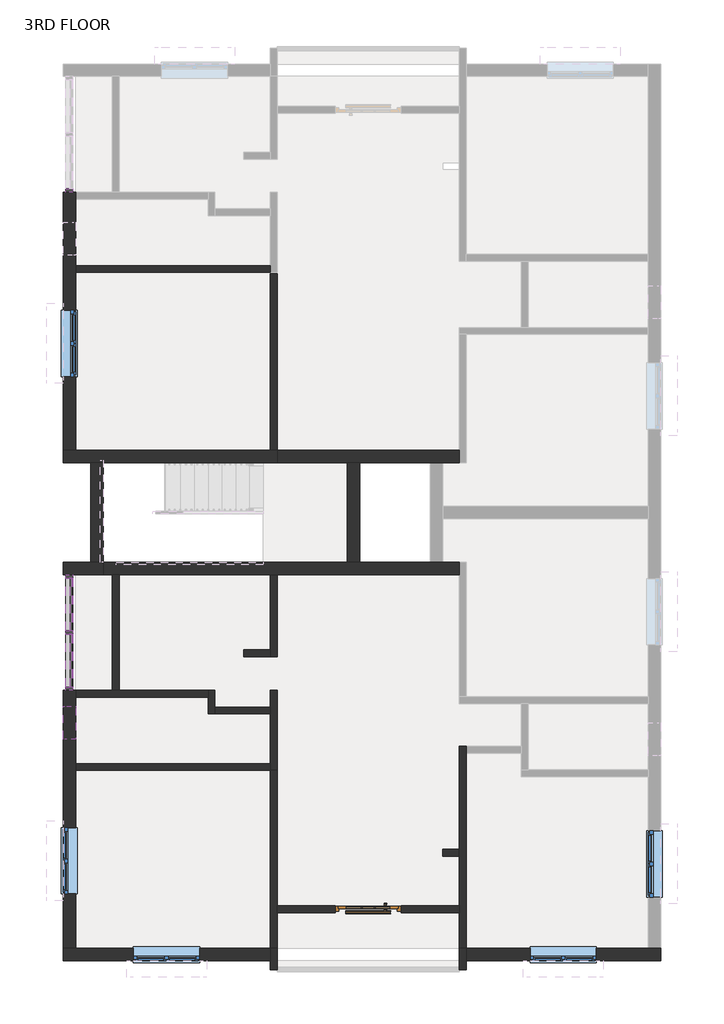
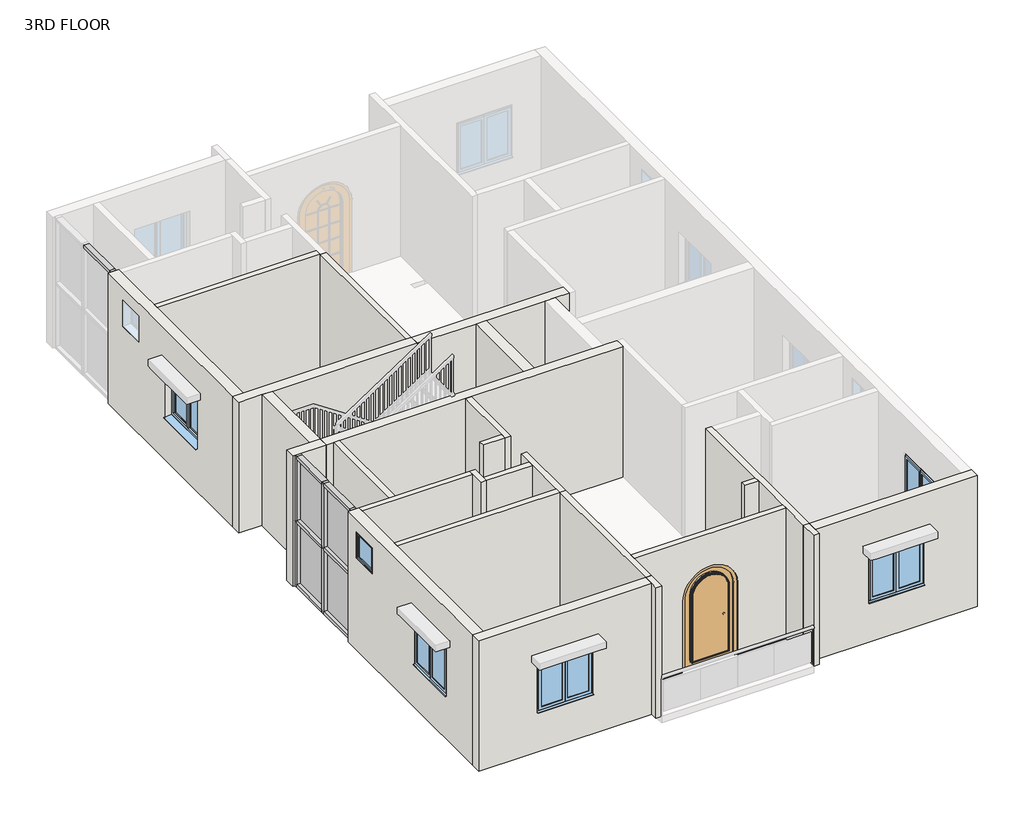
# One storey, part 1 of 4: 26 walls, 15 members, 6 windows, 4 plates, 1 door.
"""IFC4 building model written with IfcOpenShell, lengths in millimetres."""

from ifc_helpers import new_model, si_unit, point, frame, frame_2d, origin, place, context, project, spatial, polyline, circle_curve, trimmed, segment, composite_curve, outline, extrude, faceted_brep, transform, mapped, element, save
from components import door_arched_single_french_glass_wood_exterior_4_x_7_french_5c4dec95, member_801a2072, member_82905deb, member_88aa5c81, member_4491d118, system_panel_glazed_a8655be6, window_80340324, w2_windows_4_x_4_9dec5fc7

model = new_model("IFC4")

# Units and contexts
model_context = context("Model", 3, world=origin())
ifc_project = project(units=[si_unit("LENGTHUNIT", "METRE", prefix="MILLI")], contexts=[model_context])

# Site, building, storey
site = spatial("IfcSite", under=ifc_project)
building = spatial("IfcBuilding", under=site)
storey = spatial("IfcBuildingStorey", under=building, Name="3RD FLOOR", Elevation=12192.0)

# Door
placement = place(None, origin())
door_arched_single_french_glass_wood_exterior_4_x_7_french_shape = door_arched_single_french_glass_wood_exterior_4_x_7_french_5c4dec95(model_context)
element("IfcDoor", 1, ObjectType="Door_Arched_Single_French_Glass_Wood_Exterior : 4' x 7' french door", at=placement, inside=storey, context=model_context, shape_type="MappedRepresentation", body=[
    mapped(door_arched_single_french_glass_wood_exterior_4_x_7_french_shape, transform((-817.6012202, -2286.2690997, 12192.0), x_axis=(-1.0, 0.0, 0.0), y_axis=(0.0, -1.0, 0.0), z_axis=(0.0, 0.0, 1.0))),
])

# Members
member_shape = member_801a2072(model_context)
element("IfcMember", 2, ObjectType="Rectangular Mullion : 2.5\" x 5\" rectangular", at=placement, inside=storey, context=model_context, shape_type="MappedRepresentation", body=[
    mapped(member_shape, transform((-6318.2887202, 10972.5309003, 15240.0), x_axis=(0.0, 0.0, 1.0), y_axis=(-1.0, 0.0, 0.0), z_axis=(0.0, -1.0, 0.0))),
])
element("IfcMember", 3, ObjectType="Rectangular Mullion : 2.5\" x 5\" rectangular", at=placement, inside=storey, context=model_context, shape_type="MappedRepresentation", body=[
    mapped(member_shape, transform((-6318.2887202, 1803.1309003, 15240.0), x_axis=(0.0, 0.0, 1.0), y_axis=(-1.0, 0.0, 0.0), z_axis=(0.0, -1.0, 0.0))),
])
element("IfcMember", 4, ObjectType="Rectangular Mullion : 2.5\" x 5\" rectangular", at=placement, inside=storey, context=model_context, shape_type="MappedRepresentation", body=[
    mapped(member_shape, transform((-6318.2887202, 2838.1809003, 15240.0), x_axis=(0.0, 0.0, 1.0), y_axis=(-1.0, 0.0, 0.0), z_axis=(0.0, -1.0, 0.0))),
])
element("IfcMember", 5, ObjectType="Rectangular Mullion : 2.5\" x 5\" rectangular", at=placement, inside=storey, context=model_context, shape_type="MappedRepresentation", body=[
    mapped(member_shape, transform((-6318.2887202, 3809.7309003, 12192.0), x_axis=(0.0, 0.0, -1.0), y_axis=(-1.0, 0.0, 0.0), z_axis=(0.0, 1.0, 0.0))),
])
element("IfcMember", 6, ObjectType="Rectangular Mullion : 2.5\" x 5\" rectangular", at=placement, inside=storey, context=model_context, shape_type="MappedRepresentation", body=[
    mapped(member_shape, transform((-6318.2887202, 2774.6809003, 12192.0), x_axis=(0.0, 0.0, -1.0), y_axis=(-1.0, 0.0, 0.0), z_axis=(0.0, 1.0, 0.0))),
])
member_2_shape = member_82905deb(model_context)
element("IfcMember", 7, ObjectType="Rectangular Mullion : 2.5\" x 5\" rectangular", at=placement, inside=storey, context=model_context, shape_type="MappedRepresentation", body=[
    mapped(member_2_shape, transform((-6318.2887202, 2806.4309003, 12192.0), x_axis=(0.0, -1.0, 0.0), y_axis=(-1.0, 0.0, 0.0), z_axis=(0.0, 0.0, -1.0))),
])
member_3_shape = member_88aa5c81(model_context)
element("IfcMember", 8, ObjectType="Rectangular Mullion : 2.5\" x 5\" rectangular", at=placement, inside=storey, context=model_context, shape_type="MappedRepresentation", body=[
    mapped(member_3_shape, transform((-6318.2887202, 2838.1809003, 13716.0), x_axis=(0.0, 0.0, 1.0), y_axis=(-1.0, 0.0, 0.0), z_axis=(0.0, -1.0, 0.0))),
])
element("IfcMember", 9, ObjectType="Rectangular Mullion : 2.5\" x 5\" rectangular", at=placement, inside=storey, context=model_context, shape_type="MappedRepresentation", body=[
    mapped(member_3_shape, transform((-6318.2887202, 1803.1309003, 13716.0), x_axis=(0.0, 0.0, 1.0), y_axis=(-1.0, 0.0, 0.0), z_axis=(0.0, -1.0, 0.0))),
])
element("IfcMember", 10, ObjectType="Rectangular Mullion : 2.5\" x 5\" rectangular", at=placement, inside=storey, context=model_context, shape_type="MappedRepresentation", body=[
    mapped(member_2_shape, transform((-6318.2887202, 2806.4309003, 13716.0), x_axis=(0.0, -1.0, 0.0), y_axis=(-1.0, 0.0, 0.0), z_axis=(0.0, 0.0, -1.0))),
])
member_4_shape = member_4491d118(model_context)
element("IfcMember", 11, ObjectType="Rectangular Mullion : 2.5\" x 5\" rectangular", at=placement, inside=storey, context=model_context, shape_type="MappedRepresentation", body=[
    mapped(member_4_shape, transform((-6318.2887202, 10909.0309003, 12192.0), x_axis=(0.0, -1.0, 0.0), y_axis=(-1.0, 0.0, 0.0), z_axis=(0.0, 0.0, -1.0))),
])
element("IfcMember", 12, ObjectType="Rectangular Mullion : 2.5\" x 5\" rectangular", at=placement, inside=storey, context=model_context, shape_type="MappedRepresentation", body=[
    mapped(member_4_shape, transform((-6318.2887202, 1739.6309003, 12192.0), x_axis=(0.0, -1.0, 0.0), y_axis=(-1.0, 0.0, 0.0), z_axis=(0.0, 0.0, -1.0))),
])
element("IfcMember", 13, ObjectType="Rectangular Mullion : 2.5\" x 5\" rectangular", at=placement, inside=storey, context=model_context, shape_type="MappedRepresentation", body=[
    mapped(member_4_shape, transform((-6318.2887202, 3873.2309003, 15240.0), x_axis=(0.0, 1.0, 0.0), y_axis=(-1.0, 0.0, 0.0), z_axis=(0.0, 0.0, 1.0))),
])
element("IfcMember", 14, ObjectType="Rectangular Mullion : 2.5\" x 5\" rectangular", at=placement, inside=storey, context=model_context, shape_type="MappedRepresentation", body=[
    mapped(member_4_shape, transform((-6318.2887202, 10909.0309003, 13716.0), x_axis=(0.0, -1.0, 0.0), y_axis=(-1.0, 0.0, 0.0), z_axis=(0.0, 0.0, -1.0))),
])
element("IfcMember", 15, ObjectType="Rectangular Mullion : 2.5\" x 5\" rectangular", at=placement, inside=storey, context=model_context, shape_type="MappedRepresentation", body=[
    mapped(member_4_shape, transform((-6318.2887202, 1739.6309003, 13716.0), x_axis=(0.0, -1.0, 0.0), y_axis=(-1.0, 0.0, 0.0), z_axis=(0.0, 0.0, -1.0))),
])
element("IfcMember", 16, ObjectType="Rectangular Mullion : 2.5\" x 5\" rectangular", at=placement, inside=storey, context=model_context, shape_type="MappedRepresentation", body=[
    mapped(member_4_shape, transform((-6318.2887202, 3873.2309003, 13716.0), x_axis=(0.0, 1.0, 0.0), y_axis=(-1.0, 0.0, 0.0), z_axis=(0.0, 0.0, 1.0))),
])

# Plates
system_panel_glazed_shape = system_panel_glazed_a8655be6(model_context)
element("IfcPlate", 17, ObjectType="System Panel : Glazed", at=placement, inside=storey, context=model_context, shape_type="MappedRepresentation", body=[
    mapped(system_panel_glazed_shape, transform((-6318.2887202, 3323.9559003, 12255.5), x_axis=(0.0, -1.0, 0.0), y_axis=(1.0, 0.0, 0.0), z_axis=(0.0, 0.0, 1.0))),
])
element("IfcPlate", 18, ObjectType="System Panel : Glazed", at=placement, inside=storey, context=model_context, shape_type="MappedRepresentation", body=[
    mapped(system_panel_glazed_shape, transform((-6318.2887202, 2288.9059003, 12255.5), x_axis=(0.0, -1.0, 0.0), y_axis=(1.0, 0.0, 0.0), z_axis=(0.0, 0.0, 1.0))),
])
element("IfcPlate", 19, ObjectType="System Panel : Glazed", at=placement, inside=storey, context=model_context, shape_type="MappedRepresentation", body=[
    mapped(system_panel_glazed_shape, transform((-6318.2887202, 3323.9559003, 13747.75), x_axis=(0.0, -1.0, 0.0), y_axis=(1.0, 0.0, 0.0), z_axis=(0.0, 0.0, 1.0))),
])
element("IfcPlate", 20, ObjectType="System Panel : Glazed", at=placement, inside=storey, context=model_context, shape_type="MappedRepresentation", body=[
    mapped(system_panel_glazed_shape, transform((-6318.2887202, 2288.9059003, 13747.75), x_axis=(0.0, -1.0, 0.0), y_axis=(1.0, 0.0, 0.0), z_axis=(0.0, 0.0, 1.0))),
])

# Walls
element("IfcWall", 21, ObjectType="OUTER WALL 9\"", at=placement, inside=storey, context=model_context, shape_type="Brep", body=[
    faceted_brep([(-6432.5887202, -3238.7690997, 12192.0), (-2621.0012202, -3238.7690997, 12192.0), (-2621.0012202, -3238.7690997, 15240.0), (-6432.5887202, -3238.7690997, 15240.0), (-5137.1887202, -3238.7690997, 13106.4), (-5137.1887202, -3238.7690997, 14325.6), (-3917.9887202, -3238.7690997, 14325.6), (-3917.9887202, -3238.7690997, 13106.4), (-6432.5887202, -3010.1690997, 12192.0), (-6432.5887202, -3010.1690997, 15240.0), (-6203.9887202, -3010.1690997, 15240.0), (-2621.0012202, -3010.1690997, 15240.0), (-2621.0012202, -3010.1690997, 12192.0), (-6203.9887202, -3010.1690997, 12192.0), (-5137.1887202, -3010.1690997, 13106.4), (-3917.9887202, -3010.1690997, 13106.4), (-3917.9887202, -3010.1690997, 14325.6), (-5137.1887202, -3010.1690997, 14325.6)], [[[0, 1, 2, 3], [4, 5, 6, 7]], [[8, 9, 10, 11, 12, 13], [14, 15, 16, 17]], [[1, 0, 8, 13, 12]], [[3, 2, 11, 10, 9]], [[0, 3, 9, 8]], [[2, 1, 12, 11]], [[5, 4, 14, 17]], [[6, 5, 17, 16]], [[7, 6, 16, 15]], [[4, 7, 15, 14]]]),
])
element("IfcWall", 22, ObjectType="OUTER WALL 9\"", at=placement, inside=storey, context=model_context, shape_type="Brep", body=[
    faceted_brep([(-6203.9887202, -3010.1690997, 15240.0), (-6203.9887202, -3010.1690997, 12192.0), (-6203.9887202, 266.4309003, 12192.0), (-6203.9887202, 393.4309003, 12192.0), (-6203.9887202, 1612.6309003, 12192.0), (-6203.9887202, 1739.6309003, 12192.0), (-6203.9887202, 1739.6309003, 15240.0), (-6203.9887202, 1612.6309003, 15240.0), (-6203.9887202, 393.4309003, 15240.0), (-6203.9887202, 266.4309003, 15240.0), (-6203.9887202, -787.6690997, 13192.0), (-6203.9887202, -2006.8690997, 13192.0), (-6203.9887202, -2006.8690997, 14411.2), (-6203.9887202, -787.6690997, 14411.2), (-6203.9887202, 1447.5309003, 14935.2), (-6203.9887202, 1447.5309003, 14325.6), (-6203.9887202, 837.9309003, 14325.6), (-6203.9887202, 837.9309003, 14935.2), (-6432.5887202, -3010.1690997, 12192.0), (-6432.5887202, -3010.1690997, 15240.0), (-6432.5887202, 1739.6309003, 15240.0), (-6432.5887202, 1739.6309003, 12192.0), (-6432.5887202, -787.6690997, 13192.0), (-6432.5887202, -787.6690997, 14411.2), (-6432.5887202, -2006.8690997, 14411.2), (-6432.5887202, -2006.8690997, 13192.0), (-6432.5887202, 1447.5309003, 14935.2), (-6432.5887202, 837.9309003, 14935.2), (-6432.5887202, 837.9309003, 14325.6), (-6432.5887202, 1447.5309003, 14325.6)], [[[0, 1, 2, 3, 4, 5, 6, 7, 8, 9], [10, 11, 12, 13], [14, 15, 16, 17]], [[18, 19, 20, 21], [22, 23, 24, 25], [26, 27, 28, 29]], [[1, 18, 21, 5, 4, 3, 2]], [[19, 0, 9, 8, 7, 6, 20]], [[1, 0, 19, 18]], [[6, 5, 21, 20]], [[23, 22, 10, 13]], [[24, 23, 13, 12]], [[25, 24, 12, 11]], [[22, 25, 11, 10]], [[15, 14, 26, 29]], [[16, 15, 29, 28]], [[17, 16, 28, 27]], [[14, 17, 27, 26]]]),
])
element("IfcWall", 23, ObjectType="OUTER WALL 9\"", at=placement, inside=storey, context=model_context, shape_type="Brep", body=[
    faceted_brep([(4567.1987798, -3010.1690997, 12192.0), (4338.5987798, -3010.1690997, 12192.0), (985.7987798, -3010.1690997, 12192.0), (985.7987798, -3010.1690997, 15240.0), (4338.5987798, -3010.1690997, 15240.0), (4567.1987798, -3010.1690997, 15240.0), (2166.8987798, -3010.1690997, 13106.4), (3386.0987798, -3010.1690997, 13106.4), (3386.0987798, -3010.1690997, 14325.6), (2166.8987798, -3010.1690997, 14325.6), (4567.1987798, -3238.7690997, 12192.0), (4567.1987798, -3238.7690997, 15240.0), (985.7987798, -3238.7690997, 15240.0), (985.7987798, -3238.7690997, 12192.0), (2166.8987798, -3238.7690997, 13106.4), (2166.8987798, -3238.7690997, 14325.6), (3386.0987798, -3238.7690997, 14325.6), (3386.0987798, -3238.7690997, 13106.4)], [[[0, 1, 2, 3, 4, 5], [6, 7, 8, 9]], [[10, 11, 12, 13], [14, 15, 16, 17]], [[2, 1, 0, 10, 13]], [[5, 4, 3, 12, 11]], [[0, 5, 11, 10]], [[15, 14, 6, 9]], [[16, 15, 9, 8]], [[17, 16, 8, 7]], [[14, 17, 7, 6]], [[3, 2, 13, 12]]]),
])
element("IfcWall", 24, ObjectType="OUTER WALL 9\"", at=placement, inside=storey, context=model_context, shape_type="SweptSolid", body=[
    extrude(outline(polyline([(6159.2309003, 12192.0), (6159.2309003, 15240.0), (10909.0309003, 15240.0), (10909.0309003, 12192.0), (6159.2309003, 12192.0)]), holes=[polyline([(7518.1309003, 13192.0), (8737.3309003, 13192.0), (8737.3309003, 14411.2), (7518.1309003, 14411.2), (7518.1309003, 13192.0)]), polyline([(9753.3309003, 14935.2), (9753.3309003, 14325.6), (10362.9309003, 14325.6), (10362.9309003, 14935.2), (9753.3309003, 14935.2)])]), frame((-6432.5887202, 0.0, 0.0), z_axis=(1.0, 0.0, 0.0), x_axis=(0.0, 1.0, 0.0)), (0.0, 0.0, 1.0), 228.6),
])
element("IfcWall", 25, ObjectType="OUTER WALL 9\"", at=placement, inside=storey, context=model_context, shape_type="Brep", body=[
    faceted_brep([(-6432.5887202, 5930.6309003, 12192.0), (-5923.0012202, 5930.6309003, 12192.0), (-5694.4012202, 5930.6309003, 12192.0), (-2494.0012202, 5930.6309003, 12192.0), (-2494.0012202, 5930.6309003, 15240.0), (-5694.4012202, 5930.6309003, 15240.0), (-5923.0012202, 5930.6309003, 15240.0), (-6432.5887202, 5930.6309003, 15240.0), (-6432.5887202, 6159.2309003, 12192.0), (-6432.5887202, 6159.2309003, 15240.0), (-6203.9887202, 6159.2309003, 15240.0), (-2621.0012202, 6159.2309003, 15240.0), (-2494.0012202, 6159.2309003, 15240.0), (-2494.0012202, 6159.2309003, 12192.0), (-2621.0012202, 6159.2309003, 12192.0), (-6203.9887202, 6159.2309003, 12192.0)], [[[0, 1, 2, 3, 4, 5, 6, 7]], [[8, 9, 10, 11, 12, 13, 14, 15]], [[3, 2, 1, 0, 8, 15, 14, 13]], [[7, 6, 5, 4, 12, 11, 10, 9]], [[0, 7, 9, 8]], [[4, 3, 13, 12]]]),
])
element("IfcWall", 26, ObjectType="OUTER WALL 9\"", at=placement, inside=storey, context=model_context, shape_type="SweptSolid", body=[
    extrude(outline(polyline([(-5923.0012202, 4101.8309003), (-5923.0012202, 5930.6309003), (-5694.4012202, 5930.6309003), (-5694.4012202, 4101.8309003), (-5923.0012202, 4101.8309003)])), frame((0.0, 0.0, 12192.0), z_axis=(0.0, 0.0, 1.0), x_axis=(1.0, 0.0, 0.0)), (0.0, 0.0, 1.0), 3048.0),
])
element("IfcWall", 27, ObjectType="OUTER WALL 9\"", at=placement, inside=storey, context=model_context, shape_type="Brep", body=[
    faceted_brep([(-5694.4012202, 4101.8309003, 12192.0), (-5923.0012202, 4101.8309003, 12192.0), (-6432.5887202, 4101.8309003, 12192.0), (-6432.5887202, 4101.8309003, 15240.0), (-5923.0012202, 4101.8309003, 15240.0), (-5694.4012202, 4101.8309003, 15240.0), (-5694.4012202, 3873.2309003, 12192.0), (-5694.4012202, 3873.2309003, 15240.0), (-6432.5887202, 3873.2309003, 15240.0), (-6432.5887202, 3873.2309003, 12192.0)], [[[0, 1, 2, 3, 4, 5]], [[6, 7, 8, 9]], [[2, 1, 0, 6, 9]], [[5, 4, 3, 8, 7]], [[0, 5, 7, 6]], [[3, 2, 9, 8]]]),
])
element("IfcWall", 28, ObjectType="OUTER WALL 9\"", at=placement, inside=storey, context=model_context, shape_type="Brep", body=[
    faceted_brep([(-5694.4012202, 3873.2309003, 12192.0), (-5529.3012202, 3873.2309003, 12192.0), (-5402.3012202, 3873.2309003, 12192.0), (-2621.0012202, 3873.2309003, 12192.0), (-2494.0012202, 3873.2309003, 12192.0), (858.7987798, 3873.2309003, 12192.0), (858.7987798, 3873.2309003, 15240.0), (-2494.0012202, 3873.2309003, 15240.0), (-2621.0012202, 3873.2309003, 15240.0), (-5402.3012202, 3873.2309003, 15240.0), (-5529.3012202, 3873.2309003, 15240.0), (-5694.4012202, 3873.2309003, 15240.0), (-5694.4012202, 4101.8309003, 12192.0), (-5694.4012202, 4101.8309003, 15240.0), (-1198.6012202, 4101.8309003, 15240.0), (-970.0012202, 4101.8309003, 15240.0), (325.3987798, 4101.8309003, 15240.0), (553.9987798, 4101.8309003, 15240.0), (858.7987798, 4101.8309003, 15240.0), (858.7987798, 4101.8309003, 12192.0), (553.9987798, 4101.8309003, 12192.0), (325.3987798, 4101.8309003, 12192.0), (-970.0012202, 4101.8309003, 12192.0), (-1198.6012202, 4101.8309003, 12192.0)], [[[0, 1, 2, 3, 4, 5, 6, 7, 8, 9, 10, 11]], [[12, 13, 14, 15, 16, 17, 18, 19, 20, 21, 22, 23]], [[5, 4, 3, 2, 1, 0, 12, 23, 22, 21, 20, 19]], [[11, 10, 9, 8, 7, 6, 18, 17, 16, 15, 14, 13]], [[0, 11, 13, 12]], [[6, 5, 19, 18]]]),
])
element("IfcWall", 29, ObjectType="OUTER WALL 9\"", at=placement, inside=storey, context=model_context, shape_type="Brep", body=[
    faceted_brep([(858.7987798, 6159.2309003, 12192.0), (-2494.0012202, 6159.2309003, 12192.0), (-2494.0012202, 6159.2309003, 15240.0), (858.7987798, 6159.2309003, 15240.0), (858.7987798, 5930.6309003, 12192.0), (858.7987798, 5930.6309003, 15240.0), (553.9987798, 5930.6309003, 15240.0), (325.3987798, 5930.6309003, 15240.0), (-970.0012202, 5930.6309003, 15240.0), (-1198.6012202, 5930.6309003, 15240.0), (-2494.0012202, 5930.6309003, 15240.0), (-2494.0012202, 5930.6309003, 12192.0), (-1198.6012202, 5930.6309003, 12192.0), (-970.0012202, 5930.6309003, 12192.0), (325.3987798, 5930.6309003, 12192.0), (553.9987798, 5930.6309003, 12192.0)], [[[0, 1, 2, 3]], [[4, 5, 6, 7, 8, 9, 10, 11, 12, 13, 14, 15]], [[1, 0, 4, 15, 14, 13, 12, 11]], [[3, 2, 10, 9, 8, 7, 6, 5]], [[2, 1, 11, 10]], [[0, 3, 5, 4]]]),
])
element("IfcWall", 30, ObjectType="OUTER WALL 9\"", at=placement, inside=storey, context=model_context, shape_type="SweptSolid", body=[
    extrude(outline(polyline([(-1198.6012202, 4101.8309003), (-1198.6012202, 5930.6309003), (-970.0012202, 5930.6309003), (-970.0012202, 4101.8309003), (-1198.6012202, 4101.8309003)])), frame((0.0, 0.0, 12192.0), z_axis=(0.0, 0.0, 1.0), x_axis=(1.0, 0.0, 0.0)), (0.0, 0.0, 1.0), 3048.0),
])
element("IfcWall", 31, ObjectType="inner wall 5\"", at=placement, inside=storey, context=model_context, shape_type="SweptSolid", body=[
    extrude(outline(polyline([(-6202.4012202, 9562.8309003), (-2621.0012202, 9562.8309003), (-2621.0012202, 9435.8309003), (-6202.4012202, 9435.8309003), (-6202.4012202, 9562.8309003)])), frame((0.0, 0.0, 12192.0), z_axis=(0.0, 0.0, 1.0), x_axis=(1.0, 0.0, 0.0)), (0.0, 0.0, 1.0), 3048.0),
])
element("IfcWall", 32, ObjectType="inner wall 5\"", at=placement, inside=storey, context=model_context, shape_type="SweptSolid", body=[
    extrude(outline(polyline([(-5529.3012202, 1739.6309003), (-5529.3012202, 3873.2309003), (-5402.3012202, 3873.2309003), (-5402.3012202, 1739.6309003), (-5529.3012202, 1739.6309003)])), frame((0.0, 0.0, 12192.0), z_axis=(0.0, 0.0, 1.0), x_axis=(1.0, 0.0, 0.0)), (0.0, 0.0, 1.0), 3048.0),
])
element("IfcWall", 33, ObjectType="inner wall 5\"", at=placement, inside=storey, context=model_context, shape_type="Brep", body=[
    faceted_brep([(-2621.0012202, 3873.2309003, 12192.0), (-2621.0012202, 2488.9309003, 12192.0), (-2621.0012202, 2361.9309003, 12192.0), (-2621.0012202, 2361.9309003, 15240.0), (-2621.0012202, 2488.9309003, 15240.0), (-2621.0012202, 3873.2309003, 15240.0), (-2494.0012202, 3873.2309003, 12192.0), (-2494.0012202, 3873.2309003, 15240.0), (-2494.0012202, 2361.9309003, 15240.0), (-2494.0012202, 2361.9309003, 12192.0)], [[[0, 1, 2, 3, 4, 5]], [[6, 7, 8, 9]], [[2, 1, 0, 6, 9]], [[5, 4, 3, 8, 7]], [[0, 5, 7, 6]], [[3, 2, 9, 8]]]),
])
element("IfcWall", 34, ObjectType="inner wall 5\"", at=placement, inside=storey, context=model_context, shape_type="SweptSolid", body=[
    extrude(outline(polyline([(-3103.6012202, 2488.9309003), (-2621.0012202, 2488.9309003), (-2621.0012202, 2361.9309003), (-3103.6012202, 2361.9309003), (-3103.6012202, 2488.9309003)])), frame((0.0, 0.0, 12192.0), z_axis=(0.0, 0.0, 1.0), x_axis=(1.0, 0.0, 0.0)), (0.0, 0.0, 1.0), 3048.0),
])
element("IfcWall", 35, ObjectType="inner wall 5\"", at=placement, inside=storey, context=model_context, shape_type="Brep", body=[
    faceted_brep([(-6203.9887202, 1612.6309003, 12192.0), (-3764.0012202, 1612.6309003, 12192.0), (-3764.0012202, 1612.6309003, 15240.0), (-6203.9887202, 1612.6309003, 15240.0), (-6203.9887202, 1739.6309003, 12192.0), (-6203.9887202, 1739.6309003, 15240.0), (-5529.3012202, 1739.6309003, 15240.0), (-5402.3012202, 1739.6309003, 15240.0), (-3764.0012202, 1739.6309003, 15240.0), (-3764.0012202, 1739.6309003, 12192.0), (-5402.3012202, 1739.6309003, 12192.0), (-5529.3012202, 1739.6309003, 12192.0)], [[[0, 1, 2, 3]], [[4, 5, 6, 7, 8, 9, 10, 11]], [[1, 0, 4, 11, 10, 9]], [[3, 2, 8, 7, 6, 5]], [[0, 3, 5, 4]], [[2, 1, 9, 8]]]),
])
element("IfcWall", 36, ObjectType="inner wall 5\"", at=placement, inside=storey, context=model_context, shape_type="Brep", body=[
    faceted_brep([(-3764.0012202, 1739.6309003, 12192.0), (-3764.0012202, 1612.6309003, 12192.0), (-3764.0012202, 1307.8309003, 12192.0), (-3764.0012202, 1307.8309003, 15240.0), (-3764.0012202, 1612.6309003, 15240.0), (-3764.0012202, 1739.6309003, 15240.0), (-3637.0012202, 1739.6309003, 12192.0), (-3637.0012202, 1739.6309003, 15240.0), (-3637.0012202, 1434.8309003, 15240.0), (-3637.0012202, 1307.8309003, 15240.0), (-3637.0012202, 1307.8309003, 12192.0), (-3637.0012202, 1434.8309003, 12192.0)], [[[0, 1, 2, 3, 4, 5]], [[6, 7, 8, 9, 10, 11]], [[2, 1, 0, 6, 11, 10]], [[5, 4, 3, 9, 8, 7]], [[0, 5, 7, 6]], [[3, 2, 10, 9]]]),
])
element("IfcWall", 37, ObjectType="inner wall 5\"", at=placement, inside=storey, context=model_context, shape_type="SweptSolid", body=[
    extrude(outline(polyline([(-2621.0012202, 1307.8309003), (-3637.0012202, 1307.8309003), (-3637.0012202, 1434.8309003), (-2621.0012202, 1434.8309003), (-2621.0012202, 1307.8309003)])), frame((0.0, 0.0, 12192.0), z_axis=(0.0, 0.0, 1.0), x_axis=(1.0, 0.0, 0.0)), (0.0, 0.0, 1.0), 3048.0),
])
element("IfcWall", 38, ObjectType="inner wall 5\"", at=placement, inside=storey, context=model_context, shape_type="Brep", body=[
    faceted_brep([(-2621.0012202, 1739.6309003, 12192.0), (-2621.0012202, 1434.8309003, 12192.0), (-2621.0012202, 1307.8309003, 12192.0), (-2621.0012202, 393.4309003, 12192.0), (-2621.0012202, 266.4309003, 12192.0), (-2621.0012202, 266.4309003, 15240.0), (-2621.0012202, 393.4309003, 15240.0), (-2621.0012202, 1307.8309003, 15240.0), (-2621.0012202, 1434.8309003, 15240.0), (-2621.0012202, 1739.6309003, 15240.0), (-2494.0012202, 1739.6309003, 12192.0), (-2494.0012202, 1739.6309003, 15240.0), (-2494.0012202, 266.4309003, 15240.0), (-2494.0012202, 266.4309003, 12192.0)], [[[0, 1, 2, 3, 4, 5, 6, 7, 8, 9]], [[10, 11, 12, 13]], [[4, 3, 2, 1, 0, 10, 13]], [[9, 8, 7, 6, 5, 12, 11]], [[0, 9, 11, 10]], [[5, 4, 13, 12]]]),
])
element("IfcWall", 39, ObjectType="inner wall 5\"", at=placement, inside=storey, context=model_context, shape_type="SweptSolid", body=[
    extrude(outline(polyline([(-6203.9887202, 393.4309003), (-2621.0012202, 393.4309003), (-2621.0012202, 266.4309003), (-6203.9887202, 266.4309003), (-6203.9887202, 393.4309003)])), frame((0.0, 0.0, 12192.0), z_axis=(0.0, 0.0, 1.0), x_axis=(1.0, 0.0, 0.0)), (0.0, 0.0, 1.0), 3048.0),
])
element("IfcWall", 40, ObjectType="inner wall 5\"", at=placement, inside=storey, context=model_context, shape_type="Brep", body=[
    faceted_brep([(-2494.0012202, -3010.1690997, 12192.0), (-2494.0012202, -2349.7690997, 12192.0), (-2494.0012202, -2222.7690997, 12192.0), (-2494.0012202, 266.4309003, 12192.0), (-2494.0012202, 266.4309003, 15240.0), (-2494.0012202, -2222.7690997, 15240.0), (-2494.0012202, -2349.7690997, 15240.0), (-2494.0012202, -3010.1690997, 15240.0), (-2621.0012202, -3010.1690997, 12192.0), (-2621.0012202, -3010.1690997, 15240.0), (-2621.0012202, 266.4309003, 15240.0), (-2621.0012202, 266.4309003, 12192.0)], [[[0, 1, 2, 3, 4, 5, 6, 7]], [[8, 9, 10, 11]], [[3, 2, 1, 0, 8, 11]], [[7, 6, 5, 4, 10, 9]], [[4, 3, 11, 10]], [[0, 7, 9, 8]]]),
])
element("IfcWall", 41, ObjectType="inner wall 5\"", at=placement, inside=storey, context=model_context, shape_type="Brep", body=[
    faceted_brep([(985.7987798, -3010.1690997, 12192.0), (985.7987798, 583.9309003, 12192.0), (985.7987798, 710.9309003, 12192.0), (985.7987798, 710.9309003, 15240.0), (985.7987798, 583.9309003, 15240.0), (985.7987798, -3010.1690997, 15240.0), (858.7987798, -3010.1690997, 12192.0), (858.7987798, -3010.1690997, 15240.0), (858.7987798, -2349.7690997, 15240.0), (858.7987798, -2222.7690997, 15240.0), (858.7987798, -1308.3690997, 15240.0), (858.7987798, -1181.3690997, 15240.0), (858.7987798, 710.9309003, 15240.0), (858.7987798, 710.9309003, 12192.0), (858.7987798, -1181.3690997, 12192.0), (858.7987798, -1308.3690997, 12192.0), (858.7987798, -2222.7690997, 12192.0), (858.7987798, -2349.7690997, 12192.0)], [[[0, 1, 2, 3, 4, 5]], [[6, 7, 8, 9, 10, 11, 12, 13, 14, 15, 16, 17]], [[2, 1, 0, 6, 17, 16, 15, 14, 13]], [[5, 4, 3, 12, 11, 10, 9, 8, 7]], [[3, 2, 13, 12]], [[0, 5, 7, 6]]]),
])
element("IfcWall", 42, ObjectType="inner wall 5\"", at=placement, inside=storey, context=model_context, shape_type="Brep", body=[
    faceted_brep([(-2621.0012202, -3010.1690997, 12192.0), (-2621.0012202, -3238.7690997, 12192.0), (-2621.0012202, -3403.8690997, 12192.0), (-2621.0012202, -3403.8690997, 15240.0), (-2621.0012202, -3238.7690997, 15240.0), (-2621.0012202, -3010.1690997, 15240.0), (-2494.0012202, -3010.1690997, 12192.0), (-2494.0012202, -3010.1690997, 15240.0), (-2494.0012202, -3403.8690997, 15240.0), (-2494.0012202, -3403.8690997, 12192.0)], [[[0, 1, 2, 3, 4, 5]], [[6, 7, 8, 9]], [[2, 1, 0, 6, 9]], [[3, 2, 9, 8]], [[5, 4, 3, 8, 7]], [[0, 5, 7, 6]]]),
])
element("IfcWall", 43, ObjectType="inner wall 5\"", at=placement, inside=storey, context=model_context, shape_type="SweptSolid", body=[
    extrude(outline(composite_curve([segment(polyline([(12192.0, -2494.0012202), (12192.0, -1427.2012202), (13870.6, -1427.2012202)]), True, "CONTINUOUS"), segment(trimmed(circle_curve(frame_2d((13870.6, -817.6012202)), 609.6), [point((13870.6, -1427.2012202))], [point((13870.6, -208.0012202))], True, "CARTESIAN"), True, "CONTINUOUS"), segment(polyline([(13870.6, -208.0012202), (12192.0, -208.0012202), (12192.0, 858.7987798), (15240.0, 858.7987798), (15240.0, -2494.0012202), (12192.0, -2494.0012202)]), True, "CONTINUOUS")], self_intersect=False)), frame((0.0, -2349.7690997, 0.0), z_axis=(0.0, 1.0, 0.0), x_axis=(0.0, 0.0, 1.0)), (0.0, 0.0, 1.0), 127.0),
])
element("IfcWall", 44, ObjectType="inner wall 5\"", at=placement, inside=storey, context=model_context, shape_type="SweptSolid", body=[
    extrude(outline(polyline([(553.9987798, -1181.3690997), (858.7987798, -1181.3690997), (858.7987798, -1308.3690997), (553.9987798, -1308.3690997), (553.9987798, -1181.3690997)])), frame((0.0, 0.0, 12192.0), z_axis=(0.0, 0.0, 1.0), x_axis=(1.0, 0.0, 0.0)), (0.0, 0.0, 1.0), 3048.0),
])
element("IfcWall", 45, ObjectType="inner wall 5\"", at=placement, inside=storey, context=model_context, shape_type="SweptSolid", body=[
    extrude(outline(polyline([(-2621.0012202, 6159.2309003), (-2621.0012202, 9410.4309003), (-2494.0012202, 9410.4309003), (-2494.0012202, 6159.2309003), (-2621.0012202, 6159.2309003)])), frame((0.0, 0.0, 12192.0), z_axis=(0.0, 0.0, 1.0), x_axis=(1.0, 0.0, 0.0)), (0.0, 0.0, 1.0), 3048.0),
])
element("IfcWall", 46, ObjectType="inner wall 5\"", at=placement, inside=storey, context=model_context, shape_type="Brep", body=[
    faceted_brep([(858.7987798, -3010.1690997, 12192.0), (858.7987798, -3403.8690997, 12192.0), (858.7987798, -3403.8690997, 15240.0), (858.7987798, -3010.1690997, 15240.0), (985.7987798, -3010.1690997, 12192.0), (985.7987798, -3010.1690997, 15240.0), (985.7987798, -3238.7690997, 15240.0), (985.7987798, -3403.8690997, 15240.0), (985.7987798, -3403.8690997, 12192.0), (985.7987798, -3238.7690997, 12192.0)], [[[0, 1, 2, 3]], [[4, 5, 6, 7, 8, 9]], [[1, 0, 4, 9, 8]], [[2, 1, 8, 7]], [[3, 2, 7, 6, 5]], [[0, 3, 5, 4]]]),
])

# Windows
window_shape = window_80340324(model_context)
element("IfcWindow", 47, ObjectType="Fixed : 24\" x 24\"", at=placement, inside=storey, context=model_context, shape_type="MappedRepresentation", body=[
    mapped(window_shape, transform((-6318.2887202, 1180.8309003, 13411.2), x_axis=(0.0, 1.0, 0.0), y_axis=(-1.0, 0.0, 0.0), z_axis=(0.0, 0.0, 1.0))),
])
w2_windows_4_x_4_shape = w2_windows_4_x_4_9dec5fc7(model_context)
element("IfcWindow", 48, ObjectType="w2 : windows 4' x 4'", at=placement, inside=storey, context=model_context, shape_type="MappedRepresentation", body=[
    mapped(w2_windows_4_x_4_shape, transform((-4527.5887202, -3124.4690997, 12106.4), x_axis=(1.0, 0.0, 0.0), y_axis=(0.0, 1.0, 0.0), z_axis=(0.0, 0.0, 1.0))),
])
element("IfcWindow", 49, ObjectType="w2 : windows 4' x 4'", at=placement, inside=storey, context=model_context, shape_type="MappedRepresentation", body=[
    mapped(w2_windows_4_x_4_shape, transform((2776.4987798, -3124.4690997, 12106.4), x_axis=(1.0, 0.0, 0.0), y_axis=(0.0, 1.0, 0.0), z_axis=(0.0, 0.0, 1.0))),
])
element("IfcWindow", 50, ObjectType="w2 : windows 4' x 4'", at=placement, inside=storey, context=model_context, shape_type="MappedRepresentation", body=[
    mapped(w2_windows_4_x_4_shape, transform((-6318.2887202, 8127.7309003, 12192.0), x_axis=(0.0, 1.0, 0.0), y_axis=(-1.0, 0.0, 0.0), z_axis=(0.0, 0.0, 1.0))),
])
element("IfcWindow", 51, ObjectType="w2 : windows 4' x 4'", at=placement, inside=storey, context=model_context, shape_type="MappedRepresentation", body=[
    mapped(w2_windows_4_x_4_shape, transform((4452.8987798, -1454.4190997, 12192.0), x_axis=(0.0, -1.0, 0.0), y_axis=(1.0, 0.0, 0.0), z_axis=(0.0, 0.0, 1.0))),
])
element("IfcWindow", 52, ObjectType="w2 : windows 4' x 4'", at=placement, inside=storey, context=model_context, shape_type="MappedRepresentation", body=[
    mapped(w2_windows_4_x_4_shape, transform((-6318.2887202, -1397.2690997, 12192.0), x_axis=(0.0, -1.0, 0.0), y_axis=(1.0, 0.0, 0.0), z_axis=(0.0, 0.0, 1.0))),
])

save(model, "model.ifc")

# Revit data of these elements
# Type "Door_Arched_Single_French_Glass_Wood_Exterior : 4' x 7' french door"
#   Type Mark = "17"
#   Type Comments = "External Single"
#   Operation = "SingleSwingRight"
#   Keynote = "L20"
#   Analytic Construction = "<None>"
#   Wrap Layers (Int) from Ext = 0' - 6.98819"
#   Wrap Layers (Ext) from Ext = 0' - 4.03543"
#   Thickness = 0' - 1.73228"
#   Stile Shutting = 0' - 5.90551"
#   Stile - Top Rail = 0' - 5.90551"
#   Stile - Hanging = 0' - 5.90551"
#   Stile - Bottom Rail = 0' - 6.88976"
#   Rough Width = 4' - 0"
#   Rough Height = 7' - 0"
#   O/A Frame Width = 0' - 2.51969"
#   Handle Z Distance = 3' - 5.33858"
#   Glazing Thickness = 0' - 0.94488"
#   Glazing Bar Thickness = 0' - 0.7874"
#   FrameWidth = 0' - 1.65354"
#   FrameOffset - External = 0' - 0.98425"
#   FrameDepth = 0' - 3.50394"
#   Door Panel Width = 3' - 7.94488"
#   Handle X Distance = 0' - 2.95276"
#   Height = 7' - 0"
#   Structural Tolerance = 0' - 0.25591"
#   Tolerance = 0' - 0.11811"
#   Undercut = 0' - 0.15748"
#   Width = 4' - 0"
#   Door Panel Thickness = 0' - 1.73228"
#   Door Panel Height = 6' - 9.81496"
#   Cavity Closer Width = 0' - 1.9685"
#   Cavity Closer Offset from Ext = 0' - 4.03543"
#   Cavity Closer Depth = 0' - 3.34646"
#   Vis - Ironmongery = yes
#   Vis - Cavity Closers = yes
#   Define Thermal Properties by = 1
#   Material Glass = Door - Glazing
#   Handle Style = element 430241
#   Material Door = Door - Panel
#   Material Frame = BROWN
#   Material Ironmongery = Door - Handle
#   Function = (empty or 0)
#   Wall Closure = (empty or 0)
#   Assembly Code = ""
# Type "Rectangular Mullion : 2.5\" x 5\" rectangular"
#   built-in parameter 1007304 = 0.416667 (stored number, unit not read)
#   built-in parameter 1007301 = 0.104167 (stored number, unit not read)
#   built-in parameter 1007300 = 0.104167 (stored number, unit not read)
# Type "System Panel : Glazed"
#   Construction Type Id = "GSP4R"
#   Analytic Construction = "1/8 in Pilkington single glazing"
#   Visual Light Transmittance = 0.9
#   Solar Heat Gain Coefficient = 0.86
#   Heat Transfer Coefficient (U) = 1.18115 BTU/(h·ft²·°F)
#   Define Thermal Properties by = 1
# Type "OUTER WALL 9\""
#   Assembly Code = "B2010"
#   Layers, outside or top first: 0' - 9" "ROSE COLOUR" (function 1)
# Type "inner wall 5\""
#   Assembly Code = "B2010"
#   Layers, outside or top first: 0' - 5" "ROSE COLOUR" (function 1)
# Type "Fixed : 24\" x 24\""
#   Type Mark = "3"
#   Construction Type Id = "GSP4R"
#   Assembly Code = "B2020100"
#   Analytic Construction = "1/8 in Pilkington single glazing"
#   Visual Light Transmittance = 0.9
#   Solar Heat Gain Coefficient = 0.78
#   Heat Transfer Coefficient (U) = 0.6496 BTU/(h·ft²·°F)
#   Height = 2' - 0"
#   Default Sill Height = 3' - 0"
#   Width = 2' - 0"
#   Window Inset = 0' - 0 3/4"
#   Define Thermal Properties by = 1
#   Define Thermal Properties by = 1
#   Glass Pane Material = Glass
#   Sash Material = Sash
#   Wall Closure = (empty or 0)
# Type "w2 : windows 4' x 4'"
#   Type Mark = "31"
#   Operation = "DoublePanelVertical"
#   Keynote = "16.05.01"
#   Analytic Construction = "<None>"
#   Rough Width = 4' - 0"
#   Rough Height = 4' - 0"
#   Rahmentiefe = 0' - 2.3622"
#   Rahmenhöhe unten = 0' - 3.14961"
#   Rahmehöhe oben = 0' - 3.14961"
#   Rahmenbreite = 0' - 2.3622"
#   Heat Transfer Coefficient (U) = 2.81836 BTU/(h·ft²·°F)
#   Height = 4' - 0"
#   Flügeltiefe = 0' - 2.3622"
#   Flügelbreite = 0' - 2.3622"
#   Einbautiefe (von außen) [instance default] = 0' - 5.51181"
#   Width = 4' - 0"
#   Kippflügel [instance default] = yes
#   Drehflügel im Grundriß darstellen [instance default] = no
#   Drehflügel [instance default] = yes
#   Define Thermal Properties by = 1
#   Rahmen [instance default] = none
#   Glas [instance default] = blue glass
#   Flügel [instance default] = WINDOW COLOUR WHITE
#   Fensterbank aussen [instance default] = WINDOW COLOUR WHITE
#   Fensterbank innen [instance default] = WINDOW COLOUR WHITE
#   Visual Light Transmittance = 0
#   Thermal Resistance (R) = 0
#   Solar Heat Gain Coefficient = 0
#   Wall Closure = (empty or 0)
# Element 1 (IfcDoor, "Door_Arched_Single_French_Glass_Wood_Exterior : 4' x 7' french door")
#   Phase Created = New Construction
#   Materials on its faces: "Door - Panel", "Door - Handle", "BROWN", "Door - Glazing"
# Elements 2, 3, 4, 5, 6, 7, 8, 9, 10, 11, 12, 13, 14, 15, 16 (IfcMember, "Rectangular Mullion : 2.5\" x 5\" rectangular")
#   Phase Created = New Construction
#   Materials on its faces: "Aluminum"
# Elements 17, 18, 19, 20 (IfcPlate, "System Panel : Glazed")
#   Phase Created = New Construction
#   Materials on its faces: "Glass"
# Elements 21, 22, 23, 24, 25, 26, 27, 28, 29, 30 (IfcWall, "OUTER WALL 9\"")
#   Top Offset = 0' - 0"
#   Base Offset = 0' - 0"
#   wall height = 10' - 0"
#   Phase Created = New Construction
#   Base Constraint = 3RD FLOOR
#   Top Constraint = 4RTH FLOOR
#   Materials on its faces: "ROSE COLOUR"
# Elements 31, 32, 33, 34, 35, 36, 37, 38, 39, 40, 41, 42, 43, 44, 45, 46 (IfcWall, "inner wall 5\"")
#   Top Offset = 0' - 0"
#   Base Offset = 0' - 0"
#   wall height = 10' - 0"
#   Phase Created = New Construction
#   Base Constraint = 3RD FLOOR
#   Top Constraint = 4RTH FLOOR
#   Materials on its faces: "ROSE COLOUR"
# Element 47 (IfcWindow, "Fixed : 24\" x 24\"")
#   Mark = "64"
#   Phase Created = New Construction
#   Materials on its faces: "Sash", "Glass"
# Element 48 (IfcWindow, "w2 : windows 4' x 4'")
#   Mark = "56"
#   Phase Created = New Construction
#   Materials on its faces: "WINDOW COLOUR WHITE", "blue glass"
# Element 49 (IfcWindow, "w2 : windows 4' x 4'")
#   Mark = "57"
#   Phase Created = New Construction
#   Materials on its faces: "WINDOW COLOUR WHITE", "blue glass"
# Element 50 (IfcWindow, "w2 : windows 4' x 4'")
#   Mark = "60"
#   Einbautiefe (von außen) = 0' - 5.51181"
#   Kippflügel = yes
#   Drehflügel im Grundriß darstellen = no
#   Drehflügel = yes
#   Rahmen = none
#   Glas = blue glass
#   Flügel = WINDOW COLOUR WHITE
#   Fensterbank innen = WINDOW COLOUR WHITE
#   Fensterbank aussen = WINDOW COLOUR WHITE
#   Phase Created = New Construction
#   Materials on its faces: "WINDOW COLOUR WHITE", "blue glass"
# Element 51 (IfcWindow, "w2 : windows 4' x 4'")
#   Mark = "61"
#   Einbautiefe (von außen) = 0' - 5.51181"
#   Kippflügel = yes
#   Drehflügel im Grundriß darstellen = no
#   Drehflügel = yes
#   Rahmen = none
#   Glas = blue glass
#   Flügel = WINDOW COLOUR WHITE
#   Fensterbank innen = WINDOW COLOUR WHITE
#   Fensterbank aussen = WINDOW COLOUR WHITE
#   Phase Created = New Construction
#   Materials on its faces: "WINDOW COLOUR WHITE", "blue glass"
# Element 52 (IfcWindow, "w2 : windows 4' x 4'")
#   Mark = "62"
#   Einbautiefe (von außen) = 0' - 5.51181"
#   Kippflügel = yes
#   Drehflügel im Grundriß darstellen = no
#   Drehflügel = yes
#   Rahmen = none
#   Glas = blue glass
#   Flügel = WINDOW COLOUR WHITE
#   Fensterbank innen = WINDOW COLOUR WHITE
#   Fensterbank aussen = WINDOW COLOUR WHITE
#   Phase Created = New Construction
#   Materials on its faces: "WINDOW COLOUR WHITE", "blue glass"
# Materials
#   "Door - Glazing": colour RGB 218 227 224, transparency 0.85
#   "Door - Panel": class "Wood", colour RGB 210 159 95, transparency 0, Cost = 0
#   "BROWN": class "Generic", colour RGB 120 120 120, transparency 0, Cost = 0
#   "Door - Handle": colour RGB 0 0 0, transparency 0, Keynote = "P21"
#   "ROSE COLOUR": class "Generic", colour RGB 120 120 120, transparency 0, Cost = 0
#   "Glass": class "Glass", colour RGB 0 128 192, transparency 0.75, Description = "Soda Lime Glass", Cost = 0
#   "Sash": class "Wood", colour RGB 224 178 126, transparency 0, Cost = 0
#   "blue glass": class "System", colour RGB 0 0 255, transparency 0.75, Cost = 0
#   "WINDOW COLOUR WHITE": class "Generic", colour RGB 120 120 120, transparency 0, Cost = 0
#   "Aluminum": class "Metal", colour RGB 247 247 247, transparency 0, Description = "Aluminum 6061", Cost = 0
